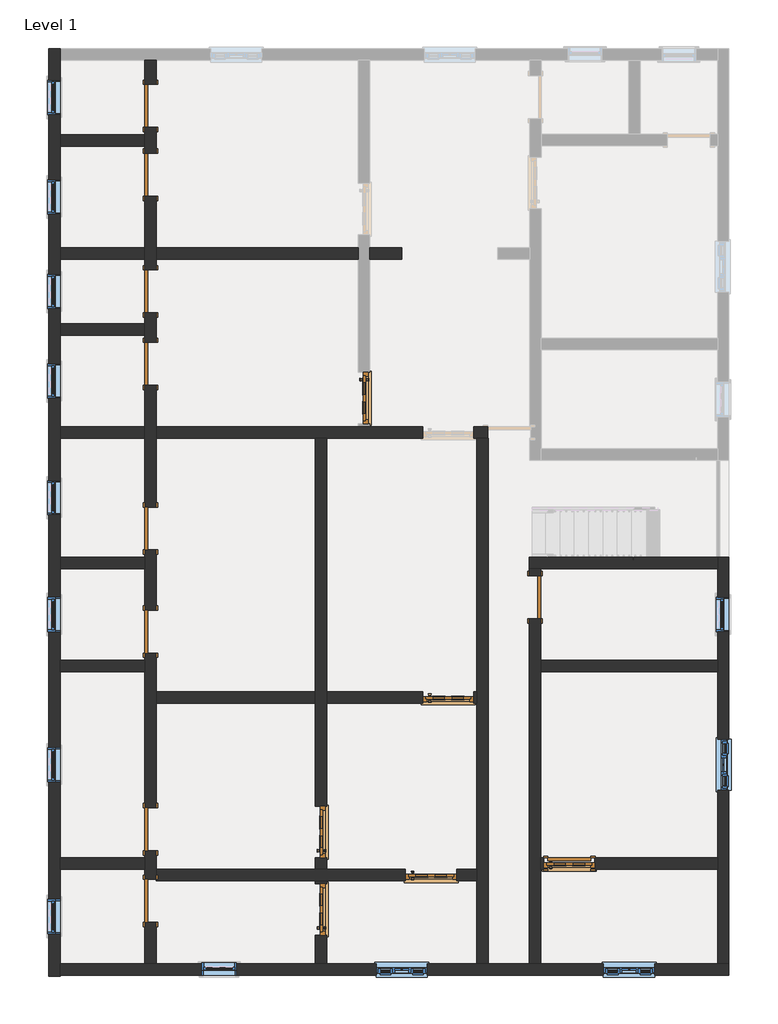
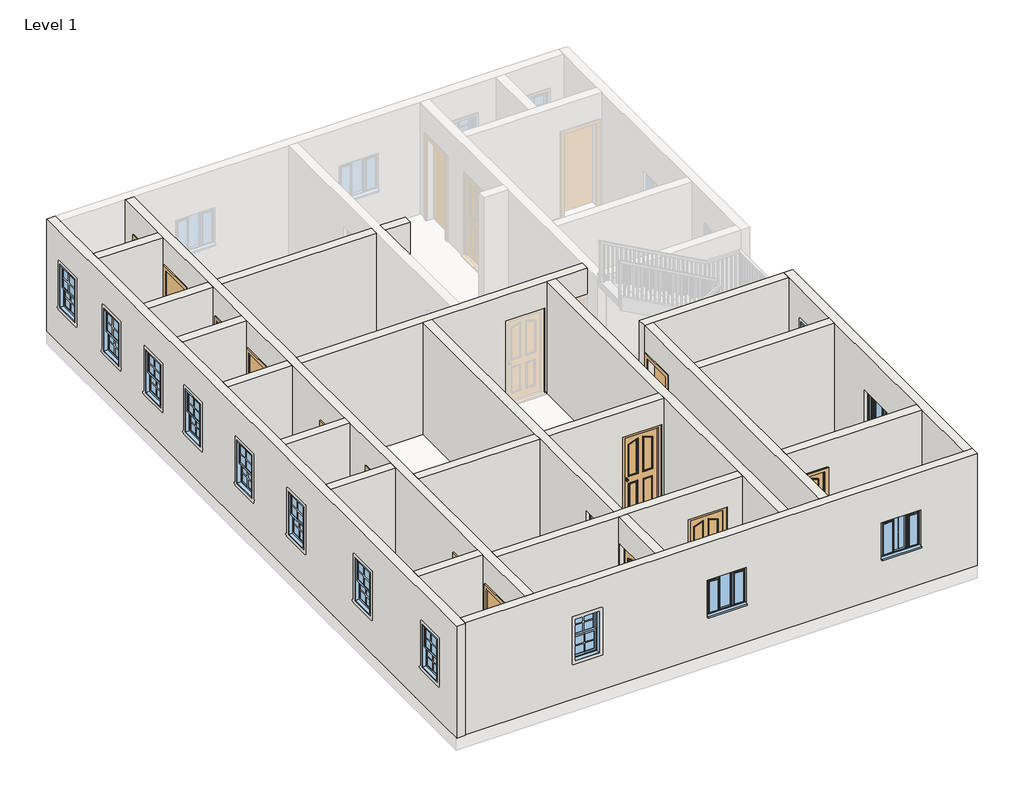
# One storey, part 1 of 3: 20 walls, 16 doors, 13 windows.
"""IFC4 building model written with IfcOpenShell, lengths in millimetres."""

from ifc_helpers import new_model, si_unit, frame, origin, origin_with_axes, place, context, project, spatial, polyline, outline, extrude, faceted_brep, transform, mapped, element, save
from components import doors_extsgl_12_910x2110mm_9a09825e, doors_extsgl_12_910x2110mm_ece77ece, door_fadea3f2, door_53b1b562, window_679d2811, windows_tpl_w_glazing_cross_bars_910x910mm_4aa0f884

model = new_model("IFC4")

# Units and contexts
model_context = context("Model", 3, world=origin())
ifc_project = project(units=[si_unit("LENGTHUNIT", "METRE", prefix="MILLI")], contexts=[model_context])

# Site, building, storey
site = spatial("IfcSite", under=ifc_project)
building = spatial("IfcBuilding", under=site)
storey = spatial("IfcBuildingStorey", under=building, Name="Level 1", Elevation=0.0)

# Doors
placement = place(None, origin())
doors_extsgl_12_910x2110mm_shape = doors_extsgl_12_910x2110mm_9a09825e(model_context)
element("IfcDoor", 1, ObjectType="Doors_ExtSgl_12 : 910x2110mm", at=placement, inside=storey, context=model_context, shape_type="MappedRepresentation", body=[
    mapped(doors_extsgl_12_910x2110mm_shape, transform((-4887.6876145, 1213.3404944, 0.0), x_axis=(0.0, -1.0, 0.0), y_axis=(1.0, 0.0, 0.0), z_axis=(0.0, 0.0, 1.0))),
])
doors_extsgl_12_910x2110mm_2_shape = doors_extsgl_12_910x2110mm_ece77ece(model_context)
element("IfcDoor", 2, ObjectType="Doors_ExtSgl_12 : 910x2110mm", at=placement, inside=storey, context=model_context, shape_type="MappedRepresentation", body=[
    mapped(doors_extsgl_12_910x2110mm_2_shape, transform((-5649.6876145, -6482.8595056, 0.0), x_axis=(0.0, 1.0, 0.0), y_axis=(-1.0, 0.0, 0.0), z_axis=(0.0, 0.0, 1.0))),
])
element("IfcDoor", 3, ObjectType="Doors_ExtSgl_12 : 910x2110mm", at=placement, inside=storey, context=model_context, shape_type="MappedRepresentation", body=[
    mapped(doors_extsgl_12_910x2110mm_2_shape, transform((-1242.7876145, -7041.6595056, 0.0), x_axis=(1.0, 0.0, 0.0), y_axis=(0.0, 1.0, 0.0), z_axis=(0.0, 0.0, 1.0))),
])
element("IfcDoor", 4, ObjectType="Doors_ExtSgl_12 : 910x2110mm", at=placement, inside=storey, context=model_context, shape_type="MappedRepresentation", body=[
    mapped(doors_extsgl_12_910x2110mm_2_shape, transform((-5649.6876145, -7854.4595056, 0.0), x_axis=(0.0, 1.0, 0.0), y_axis=(-1.0, 0.0, 0.0), z_axis=(0.0, 0.0, 1.0))),
])
element("IfcDoor", 5, ObjectType="Doors_ExtSgl_12 : 910x2110mm", at=placement, inside=storey, context=model_context, shape_type="MappedRepresentation", body=[
    mapped(doors_extsgl_12_910x2110mm_2_shape, transform((-3693.8876145, -7244.8595056, 0.0), x_axis=(1.0, 0.0, 0.0), y_axis=(0.0, 1.0, 0.0), z_axis=(0.0, 0.0, 1.0))),
])
element("IfcDoor", 6, ObjectType="Doors_ExtSgl_12 : 910x2110mm", at=placement, inside=storey, context=model_context, shape_type="MappedRepresentation", body=[
    mapped(doors_extsgl_12_910x2110mm_2_shape, transform((-3389.0876145, -4095.2595056, 0.0), x_axis=(1.0, 0.0, 0.0), y_axis=(0.0, 1.0, 0.0), z_axis=(0.0, 0.0, 1.0))),
])
door_shape = door_fadea3f2(model_context)
element("IfcDoor", 7, ObjectType="Single-Flush : 30\" x 80\"", at=placement, inside=storey, context=model_context, shape_type="MappedRepresentation", body=[
    mapped(door_shape, transform((-8672.2876145, 5175.7404944, 0.0), x_axis=(0.0, 1.0, 0.0), y_axis=(-1.0, 0.0, 0.0), z_axis=(0.0, 0.0, 1.0))),
])
element("IfcDoor", 8, ObjectType="Single-Flush : 30\" x 80\"", at=placement, inside=storey, context=model_context, shape_type="MappedRepresentation", body=[
    mapped(door_shape, transform((-8672.2876145, -7702.0595056, 0.0), x_axis=(0.0, 1.0, 0.0), y_axis=(-1.0, 0.0, 0.0), z_axis=(0.0, 0.0, 1.0))),
])
element("IfcDoor", 9, ObjectType="Single-Flush : 30\" x 80\"", at=placement, inside=storey, context=model_context, shape_type="MappedRepresentation", body=[
    mapped(door_shape, transform((-1852.3876145, -2317.2595056, 0.0), x_axis=(0.0, -1.0, 0.0), y_axis=(1.0, 0.0, 0.0), z_axis=(0.0, 0.0, 1.0))),
])
element("IfcDoor", 10, ObjectType="Single-Flush : 30\" x 80\"", at=placement, inside=storey, context=model_context, shape_type="MappedRepresentation", body=[
    mapped(door_shape, transform((-1242.7876145, -7041.6595056, 0.0), x_axis=(1.0, 0.0, 0.0), y_axis=(0.0, 1.0, 0.0), z_axis=(0.0, 0.0, 1.0))),
])
door_2_shape = door_53b1b562(model_context)
element("IfcDoor", 11, ObjectType="Single-Flush : 30\" x 80\"", at=placement, inside=storey, context=model_context, shape_type="MappedRepresentation", body=[
    mapped(door_2_shape, transform((-8672.2876145, 6394.9404944, 0.0), x_axis=(0.0, -1.0, 0.0), y_axis=(1.0, 0.0, 0.0), z_axis=(0.0, 0.0, 1.0))),
])
element("IfcDoor", 12, ObjectType="Single-Flush : 30\" x 80\"", at=placement, inside=storey, context=model_context, shape_type="MappedRepresentation", body=[
    mapped(door_2_shape, transform((-8672.2876145, 3105.6404944, 0.0), x_axis=(0.0, -1.0, 0.0), y_axis=(1.0, 0.0, 0.0), z_axis=(0.0, 0.0, 1.0))),
])
element("IfcDoor", 13, ObjectType="Single-Flush : 30\" x 80\"", at=placement, inside=storey, context=model_context, shape_type="MappedRepresentation", body=[
    mapped(door_2_shape, transform((-8672.2876145, 1822.9404944, 0.0), x_axis=(0.0, -1.0, 0.0), y_axis=(1.0, 0.0, 0.0), z_axis=(0.0, 0.0, 1.0))),
])
element("IfcDoor", 14, ObjectType="Single-Flush : 30\" x 80\"", at=placement, inside=storey, context=model_context, shape_type="MappedRepresentation", body=[
    mapped(door_2_shape, transform((-8672.2876145, -1098.0595056, 0.0), x_axis=(0.0, -1.0, 0.0), y_axis=(1.0, 0.0, 0.0), z_axis=(0.0, 0.0, 1.0))),
])
element("IfcDoor", 15, ObjectType="Single-Flush : 30\" x 80\"", at=placement, inside=storey, context=model_context, shape_type="MappedRepresentation", body=[
    mapped(door_2_shape, transform((-8672.2876145, -2926.8595056, 0.0), x_axis=(0.0, -1.0, 0.0), y_axis=(1.0, 0.0, 0.0), z_axis=(0.0, 0.0, 1.0))),
])
element("IfcDoor", 16, ObjectType="Single-Flush : 30\" x 80\"", at=placement, inside=storey, context=model_context, shape_type="MappedRepresentation", body=[
    mapped(door_2_shape, transform((-8672.2876145, -6432.0595056, 0.0), x_axis=(0.0, -1.0, 0.0), y_axis=(1.0, 0.0, 0.0), z_axis=(0.0, 0.0, 1.0))),
])

# Walls
element("IfcWall", 17, ObjectType="4.5\"", at=placement, inside=storey, context=model_context, shape_type="Brep", body=[
    faceted_brep([(-8773.8876145, -6813.0595056, 0.0), (-8773.8876145, -6940.0595056, 0.0), (-8773.8876145, -7143.2595056, 0.0), (-8773.8876145, -7321.0595056, 0.0), (-8773.8876145, -7321.0595056, 2032.0), (-8773.8876145, -8083.0595056, 2032.0), (-8773.8876145, -8083.0595056, 0.0), (-8773.8876145, -8819.6595056, 0.0), (-8773.8876145, -8819.6595056, 2743.2), (-8773.8876145, -7143.2595056, 2743.2), (-8773.8876145, -6940.0595056, 2743.2), (-8773.8876145, -3638.0595056, 2743.2), (-8773.8876145, -3434.8595056, 2743.2), (-8773.8876145, -1809.2595056, 2743.2), (-8773.8876145, -1606.0595056, 2743.2), (-8773.8876145, 502.1404944, 2743.2), (-8773.8876145, 705.3404944, 2743.2), (-8773.8876145, 2330.9404944, 2743.2), (-8773.8876145, 2534.1404944, 2743.2), (-8773.8876145, 3677.1404944, 2743.2), (-8773.8876145, 3880.3404944, 2743.2), (-8773.8876145, 5683.7404944, 2743.2), (-8773.8876145, 5886.9404944, 2743.2), (-8773.8876145, 7207.7404944, 2743.2), (-8773.8876145, 7207.7404944, 0.0), (-8773.8876145, 6775.9404944, 0.0), (-8773.8876145, 6775.9404944, 2032.0), (-8773.8876145, 6013.9404944, 2032.0), (-8773.8876145, 6013.9404944, 0.0), (-8773.8876145, 5886.9404944, 0.0), (-8773.8876145, 5683.7404944, 0.0), (-8773.8876145, 5556.7404944, 0.0), (-8773.8876145, 5556.7404944, 2032.0), (-8773.8876145, 4794.7404944, 2032.0), (-8773.8876145, 4794.7404944, 0.0), (-8773.8876145, 3880.3404944, 0.0), (-8773.8876145, 3677.1404944, 0.0), (-8773.8876145, 3486.6404944, 0.0), (-8773.8876145, 3486.6404944, 2032.0), (-8773.8876145, 2724.6404944, 2032.0), (-8773.8876145, 2724.6404944, 0.0), (-8773.8876145, 2534.1404944, 0.0), (-8773.8876145, 2330.9404944, 0.0), (-8773.8876145, 2203.9404944, 0.0), (-8773.8876145, 2203.9404944, 2032.0), (-8773.8876145, 1441.9404944, 2032.0), (-8773.8876145, 1441.9404944, 0.0), (-8773.8876145, 705.3404944, 0.0), (-8773.8876145, 502.1404944, 0.0), (-8773.8876145, -717.0595056, 0.0), (-8773.8876145, -717.0595056, 2032.0), (-8773.8876145, -1479.0595056, 2032.0), (-8773.8876145, -1479.0595056, 0.0), (-8773.8876145, -1606.0595056, 0.0), (-8773.8876145, -1809.2595056, 0.0), (-8773.8876145, -2545.8595056, 0.0), (-8773.8876145, -2545.8595056, 2032.0), (-8773.8876145, -3307.8595056, 2032.0), (-8773.8876145, -3307.8595056, 0.0), (-8773.8876145, -3434.8595056, 0.0), (-8773.8876145, -3638.0595056, 0.0), (-8773.8876145, -6051.0595056, 0.0), (-8773.8876145, -6051.0595056, 2032.0), (-8773.8876145, -6813.0595056, 2032.0), (-8570.6876145, -7321.0595056, 2032.0), (-8570.6876145, -7321.0595056, 0.0), (-8570.6876145, -7143.2595056, 0.0), (-8570.6876145, -6813.0595056, 0.0), (-8570.6876145, -6813.0595056, 2032.0), (-8570.6876145, -6051.0595056, 2032.0), (-8570.6876145, -6051.0595056, 0.0), (-8570.6876145, -4196.8595056, 0.0), (-8570.6876145, -3993.6595056, 0.0), (-8570.6876145, -3307.8595056, 0.0), (-8570.6876145, -3307.8595056, 2032.0), (-8570.6876145, -2545.8595056, 2032.0), (-8570.6876145, -2545.8595056, 0.0), (-8570.6876145, -1479.0595056, 0.0), (-8570.6876145, -1479.0595056, 2032.0), (-8570.6876145, -717.0595056, 2032.0), (-8570.6876145, -717.0595056, 0.0), (-8570.6876145, 502.1404944, 0.0), (-8570.6876145, 705.3404944, 0.0), (-8570.6876145, 1441.9404944, 0.0), (-8570.6876145, 1441.9404944, 2032.0), (-8570.6876145, 2203.9404944, 2032.0), (-8570.6876145, 2203.9404944, 0.0), (-8570.6876145, 2724.6404944, 0.0), (-8570.6876145, 2724.6404944, 2032.0), (-8570.6876145, 3486.6404944, 2032.0), (-8570.6876145, 3486.6404944, 0.0), (-8570.6876145, 3677.1404944, 0.0), (-8570.6876145, 3880.3404944, 0.0), (-8570.6876145, 4794.7404944, 0.0), (-8570.6876145, 4794.7404944, 2032.0), (-8570.6876145, 5556.7404944, 2032.0), (-8570.6876145, 5556.7404944, 0.0), (-8570.6876145, 6013.9404944, 0.0), (-8570.6876145, 6013.9404944, 2032.0), (-8570.6876145, 6775.9404944, 2032.0), (-8570.6876145, 6775.9404944, 0.0), (-8570.6876145, 7207.7404944, 0.0), (-8570.6876145, 7207.7404944, 2743.2), (-8570.6876145, 3880.3404944, 2743.2), (-8570.6876145, 3677.1404944, 2743.2), (-8570.6876145, 705.3404944, 2743.2), (-8570.6876145, 502.1404944, 2743.2), (-8570.6876145, -3993.6595056, 2743.2), (-8570.6876145, -4196.8595056, 2743.2), (-8570.6876145, -7143.2595056, 2743.2), (-8570.6876145, -7346.4595056, 2743.2), (-8570.6876145, -8819.6595056, 2743.2), (-8570.6876145, -8819.6595056, 0.0), (-8570.6876145, -8083.0595056, 0.0), (-8570.6876145, -8083.0595056, 2032.0)], [[[0, 1, 2, 3, 4, 5, 6, 7, 8, 9, 10, 11, 12, 13, 14, 15, 16, 17, 18, 19, 20, 21, 22, 23, 24, 25, 26, 27, 28, 29, 30, 31, 32, 33, 34, 35, 36, 37, 38, 39, 40, 41, 42, 43, 44, 45, 46, 47, 48, 49, 50, 51, 52, 53, 54, 55, 56, 57, 58, 59, 60, 61, 62, 63]], [[64, 65, 66, 67, 68, 69, 70, 71, 72, 73, 74, 75, 76, 77, 78, 79, 80, 81, 82, 83, 84, 85, 86, 87, 88, 89, 90, 91, 92, 93, 94, 95, 96, 97, 98, 99, 100, 101, 102, 103, 104, 105, 106, 107, 108, 109, 110, 111, 112, 113, 114]], [[25, 24, 101, 100]], [[97, 96, 31, 30, 29, 28]], [[37, 36, 35, 34, 93, 92, 91, 90]], [[43, 42, 41, 40, 87, 86]], [[49, 48, 47, 46, 83, 82, 81, 80]], [[55, 54, 53, 52, 77, 76]], [[61, 60, 59, 58, 73, 72, 71, 70]], [[113, 112, 7, 6]], [[67, 66, 65, 3, 2, 1, 0]], [[8, 7, 112, 111]], [[24, 23, 102, 101]], [[98, 97, 28, 27]], [[99, 98, 27, 26]], [[100, 99, 26, 25]], [[32, 31, 96, 95]], [[33, 32, 95, 94]], [[34, 33, 94, 93]], [[88, 87, 40, 39]], [[89, 88, 39, 38]], [[90, 89, 38, 37]], [[84, 83, 46, 45]], [[85, 84, 45, 44]], [[86, 85, 44, 43]], [[78, 77, 52, 51]], [[79, 78, 51, 50]], [[80, 79, 50, 49]], [[74, 73, 58, 57]], [[75, 74, 57, 56]], [[76, 75, 56, 55]], [[68, 67, 0, 63]], [[69, 68, 63, 62]], [[70, 69, 62, 61]], [[4, 3, 65, 64]], [[5, 4, 64, 114]], [[6, 5, 114, 113]], [[23, 22, 21, 20, 19, 18, 17, 16, 15, 14, 13, 12, 11, 10, 9, 8, 111, 110, 109, 108, 107, 106, 105, 104, 103, 102]]]),
])
element("IfcWall", 18, ObjectType="4.5\"", at=placement, inside=storey, context=model_context, shape_type="SweptSolid", body=[
    extrude(outline(polyline([(-8773.8876145, 5683.7404944), (-10272.4876145, 5683.7404944), (-10272.4876145, 5886.9404944), (-8773.8876145, 5886.9404944), (-8773.8876145, 5683.7404944)])), origin_with_axes(), (0.0, 0.0, 1.0), 2743.2),
])
element("IfcWall", 19, ObjectType="4.5\"", at=placement, inside=storey, context=model_context, shape_type="SweptSolid", body=[
    extrude(outline(polyline([(-8773.8876145, 3677.1404944), (-10272.4876145, 3677.1404944), (-10272.4876145, 3880.3404944), (-8773.8876145, 3880.3404944), (-8773.8876145, 3677.1404944)])), origin_with_axes(), (0.0, 0.0, 1.0), 2743.2),
])
element("IfcWall", 20, ObjectType="4.5\"", at=placement, inside=storey, context=model_context, shape_type="SweptSolid", body=[
    extrude(outline(polyline([(-8773.8876145, 2330.9404944), (-10272.4876145, 2330.9404944), (-10272.4876145, 2534.1404944), (-8773.8876145, 2534.1404944), (-8773.8876145, 2330.9404944)])), origin_with_axes(), (0.0, 0.0, 1.0), 2743.2),
])
element("IfcWall", 21, ObjectType="4.5\"", at=placement, inside=storey, context=model_context, shape_type="Brep", body=[
    faceted_brep([(-10272.4876145, 502.1404944, 2743.2), (-10272.4876145, 502.1404944, 0.0), (-8773.8876145, 502.1404944, 0.0), (-8773.8876145, 502.1404944, 2743.2), (-10272.4876145, 705.3404944, 0.0), (-10272.4876145, 705.3404944, 2743.2), (-8773.8876145, 705.3404944, 2743.2), (-8773.8876145, 705.3404944, 0.0)], [[[0, 1, 2, 3]], [[4, 5, 6, 7]], [[1, 4, 7, 2]], [[1, 0, 5, 4]], [[3, 2, 7, 6]], [[5, 0, 3, 6]]]),
    faceted_brep([(-1941.2876145, 502.1404944, 2032.0), (-1941.2876145, 502.1404944, 2743.2), (-2677.8876145, 502.1404944, 2743.2), (-2881.0876145, 502.1404944, 2743.2), (-5548.0876145, 502.1404944, 2743.2), (-5751.2876145, 502.1404944, 2743.2), (-8570.6876145, 502.1404944, 2743.2), (-8570.6876145, 502.1404944, 0.0), (-5751.2876145, 502.1404944, 0.0), (-5548.0876145, 502.1404944, 0.0), (-3844.0876145, 502.1404944, 0.0), (-3844.0876145, 502.1404944, 2110.0), (-2934.0876145, 502.1404944, 2110.0), (-2934.0876145, 502.1404944, 0.0), (-2881.0876145, 502.1404944, 0.0), (-2690.5876145, 502.1404944, 0.0), (-2690.5876145, 502.1404944, 2032.0), (-1941.2876145, 705.3404944, 2743.2), (-1941.2876145, 705.3404944, 2032.0), (-2690.5876145, 705.3404944, 2032.0), (-2690.5876145, 705.3404944, 0.0), (-2934.0876145, 705.3404944, 0.0), (-2934.0876145, 705.3404944, 2110.0), (-3844.0876145, 705.3404944, 2110.0), (-3844.0876145, 705.3404944, 0.0), (-4786.0876145, 705.3404944, 0.0), (-4989.2876145, 705.3404944, 0.0), (-8570.6876145, 705.3404944, 0.0), (-8570.6876145, 705.3404944, 2743.2), (-4989.2876145, 705.3404944, 2743.2), (-4786.0876145, 705.3404944, 2743.2)], [[[0, 1, 2, 3, 4, 5, 6, 7, 8, 9, 10, 11, 12, 13, 14, 15, 16]], [[17, 18, 19, 20, 21, 22, 23, 24, 25, 26, 27, 28, 29, 30]], [[20, 15, 14, 13, 21]], [[24, 10, 9, 8, 7, 27, 26, 25]], [[7, 6, 28, 27]], [[1, 0, 18, 17]], [[16, 19, 18, 0]], [[19, 16, 15, 20]], [[24, 23, 11, 10]], [[22, 21, 13, 12]], [[23, 22, 12, 11]], [[1, 17, 30, 29, 28, 6, 5, 4, 3, 2]]]),
])
element("IfcWall", 22, ObjectType="4.5\"", at=placement, inside=storey, context=model_context, shape_type="SweptSolid", body=[
    extrude(outline(polyline([(-8773.8876145, -1809.2595056), (-10272.4876145, -1809.2595056), (-10272.4876145, -1606.0595056), (-8773.8876145, -1606.0595056), (-8773.8876145, -1809.2595056)])), origin_with_axes(), (0.0, 0.0, 1.0), 2743.2),
])
element("IfcWall", 23, ObjectType="4.5\"", at=placement, inside=storey, context=model_context, shape_type="SweptSolid", body=[
    extrude(outline(polyline([(-8773.8876145, -3638.0595056), (-10272.4876145, -3638.0595056), (-10272.4876145, -3434.8595056), (-8773.8876145, -3434.8595056), (-8773.8876145, -3638.0595056)])), origin_with_axes(), (0.0, 0.0, 1.0), 2743.2),
])
element("IfcWall", 24, ObjectType="4.5\"", at=placement, inside=storey, context=model_context, shape_type="SweptSolid", body=[
    extrude(outline(polyline([(-8773.8876145, -7143.2595056), (-10272.4876145, -7143.2595056), (-10272.4876145, -6940.0595056), (-8773.8876145, -6940.0595056), (-8773.8876145, -7143.2595056)])), origin_with_axes(), (0.0, 0.0, 1.0), 2743.2),
])
element("IfcWall", 25, ObjectType="4.5\"", at=placement, inside=storey, context=model_context, shape_type="Brep", body=[
    faceted_brep([(-3238.8876145, -7346.4595056, 2110.0), (-3238.8876145, -7346.4595056, 0.0), (-2881.0876145, -7346.4595056, 0.0), (-2881.0876145, -7346.4595056, 2743.2), (-5548.0876145, -7346.4595056, 2743.2), (-5751.2876145, -7346.4595056, 2743.2), (-8570.6876145, -7346.4595056, 2743.2), (-8570.6876145, -7346.4595056, 0.0), (-5751.2876145, -7346.4595056, 0.0), (-5548.0876145, -7346.4595056, 0.0), (-4148.8876145, -7346.4595056, 0.0), (-4148.8876145, -7346.4595056, 2110.0), (-2881.0876145, -7143.2595056, 0.0), (-3238.8876145, -7143.2595056, 0.0), (-3238.8876145, -7143.2595056, 2110.0), (-4148.8876145, -7143.2595056, 2110.0), (-4148.8876145, -7143.2595056, 0.0), (-5548.0876145, -7143.2595056, 0.0), (-5751.2876145, -7143.2595056, 0.0), (-8570.6876145, -7143.2595056, 0.0), (-8570.6876145, -7143.2595056, 2743.2), (-5751.2876145, -7143.2595056, 2743.2), (-5548.0876145, -7143.2595056, 2743.2), (-2881.0876145, -7143.2595056, 2743.2), (-8570.6876145, -7321.0595056, 0.0)], [[[0, 1, 2, 3, 4, 5, 6, 7, 8, 9, 10, 11]], [[12, 13, 14, 15, 16, 17, 18, 19, 20, 21, 22, 23]], [[2, 1, 13, 12]], [[10, 9, 8, 7, 24, 19, 18, 17, 16]], [[7, 6, 20, 19, 24]], [[3, 2, 12, 23]], [[16, 15, 11, 10]], [[14, 13, 1, 0]], [[15, 14, 0, 11]], [[6, 5, 4, 3, 23, 22, 21, 20]]]),
])
element("IfcWall", 26, ObjectType="4.5\"", at=placement, inside=storey, context=model_context, shape_type="Brep", body=[
    faceted_brep([(-5751.2876145, -8819.6595056, 0.0), (-5751.2876145, -8819.6595056, 2743.2), (-5751.2876145, -7346.4595056, 2743.2), (-5751.2876145, -7346.4595056, 0.0), (-5751.2876145, -7399.4595056, 0.0), (-5751.2876145, -7399.4595056, 2110.0), (-5751.2876145, -8309.4595056, 2110.0), (-5751.2876145, -8309.4595056, 0.0), (-5548.0876145, -8819.6595056, 2743.2), (-5548.0876145, -8819.6595056, 0.0), (-5548.0876145, -8309.4595056, 0.0), (-5548.0876145, -8309.4595056, 2110.0), (-5548.0876145, -7399.4595056, 2110.0), (-5548.0876145, -7399.4595056, 0.0), (-5548.0876145, -7346.4595056, 0.0), (-5548.0876145, -7346.4595056, 2743.2)], [[[0, 1, 2, 3, 4, 5, 6, 7]], [[8, 9, 10, 11, 12, 13, 14, 15]], [[9, 0, 7, 10]], [[13, 4, 3, 14]], [[1, 0, 9, 8]], [[3, 2, 15, 14]], [[7, 6, 11, 10]], [[5, 4, 13, 12]], [[6, 5, 12, 11]], [[1, 8, 15, 2]]]),
    faceted_brep([(-5751.2876145, 502.1404944, 2743.2), (-5751.2876145, 502.1404944, 0.0), (-5751.2876145, -3993.6595056, 0.0), (-5751.2876145, -4196.8595056, 0.0), (-5751.2876145, -6027.8595056, 0.0), (-5751.2876145, -6027.8595056, 2110.0), (-5751.2876145, -6937.8595056, 2110.0), (-5751.2876145, -6937.8595056, 0.0), (-5751.2876145, -7143.2595056, 0.0), (-5751.2876145, -7143.2595056, 2743.2), (-5751.2876145, -4196.8595056, 2743.2), (-5751.2876145, -3993.6595056, 2743.2), (-5548.0876145, 502.1404944, 0.0), (-5548.0876145, 502.1404944, 2743.2), (-5548.0876145, -3993.6595056, 2743.2), (-5548.0876145, -4196.8595056, 2743.2), (-5548.0876145, -7143.2595056, 2743.2), (-5548.0876145, -7143.2595056, 0.0), (-5548.0876145, -6937.8595056, 0.0), (-5548.0876145, -6937.8595056, 2110.0), (-5548.0876145, -6027.8595056, 2110.0), (-5548.0876145, -6027.8595056, 0.0), (-5548.0876145, -4196.8595056, 0.0), (-5548.0876145, -3993.6595056, 0.0)], [[[0, 1, 2, 3, 4, 5, 6, 7, 8, 9, 10, 11]], [[12, 13, 14, 15, 16, 17, 18, 19, 20, 21, 22, 23]], [[1, 12, 23, 22, 21, 4, 3, 2]], [[7, 18, 17, 8]], [[1, 0, 13, 12]], [[9, 8, 17, 16]], [[7, 6, 19, 18]], [[5, 4, 21, 20]], [[6, 5, 20, 19]], [[13, 0, 11, 10, 9, 16, 15, 14]]]),
])
element("IfcWall", 27, ObjectType="4.5\"", at=placement, inside=storey, context=model_context, shape_type="SweptSolid", body=[
    extrude(outline(polyline([(-8570.6876145, -4196.8595056), (-8570.6876145, -3993.6595056), (-5751.2876145, -3993.6595056), (-5751.2876145, -4196.8595056), (-8570.6876145, -4196.8595056)])), origin_with_axes(), (0.0, 0.0, 1.0), 2743.2),
    extrude(outline(polyline([(0.0, -2881.0876145), (2743.2, -2881.0876145), (2743.2, -5548.0876145), (0.0, -5548.0876145), (0.0, -3844.0876145), (2110.0, -3844.0876145), (2110.0, -2934.0876145), (0.0, -2934.0876145), (0.0, -2881.0876145)])), frame((0.0, -4196.8595056, 0.0), z_axis=(0.0, 1.0, 0.0), x_axis=(0.0, 0.0, 1.0)), (0.0, 0.0, 1.0), 203.2),
])
element("IfcWall", 28, ObjectType="4.5\"", at=placement, inside=storey, context=model_context, shape_type="Brep", body=[
    faceted_brep([(-2881.0876145, 502.1404944, 0.0), (-2881.0876145, -3993.6595056, 0.0), (-2881.0876145, -4196.8595056, 0.0), (-2881.0876145, -7143.2595056, 0.0), (-2881.0876145, -7346.4595056, 0.0), (-2881.0876145, -8819.6595056, 0.0), (-2881.0876145, -8819.6595056, 2743.2), (-2881.0876145, -7346.4595056, 2743.2), (-2881.0876145, -7143.2595056, 2743.2), (-2881.0876145, -4196.8595056, 2743.2), (-2881.0876145, -3993.6595056, 2743.2), (-2881.0876145, 502.1404944, 2743.2), (-2677.8876145, 502.1404944, 0.0), (-2677.8876145, 502.1404944, 2743.2), (-2677.8876145, -8819.6595056, 2743.2), (-2677.8876145, -8819.6595056, 0.0), (-2690.5876145, 502.1404944, 0.0)], [[[0, 1, 2, 3, 4, 5, 6, 7, 8, 9, 10, 11]], [[12, 13, 14, 15]], [[5, 4, 3, 2, 1, 0, 16, 12, 15]], [[6, 5, 15, 14]], [[0, 11, 13, 12, 16]], [[11, 10, 9, 8, 7, 6, 14, 13]]]),
])
element("IfcWall", 29, ObjectType="4.5\"", at=placement, inside=storey, context=model_context, shape_type="SweptSolid", body=[
    extrude(outline(polyline([(-4214.5876145, 3880.3404944), (-4214.5876145, 3677.1404944), (-4786.0876145, 3677.1404944), (-4786.0876145, 3880.3404944), (-4214.5876145, 3880.3404944)])), origin_with_axes(), (0.0, 0.0, 1.0), 2743.2),
    extrude(outline(polyline([(-8570.6876145, 3677.1404944), (-8570.6876145, 3880.3404944), (-4989.2876145, 3880.3404944), (-4989.2876145, 3677.1404944), (-8570.6876145, 3677.1404944)])), origin_with_axes(), (0.0, 0.0, 1.0), 2743.2),
])
element("IfcWall", 30, ObjectType="4.5\"", at=placement, inside=storey, context=model_context, shape_type="Brep", body=[
    faceted_brep([(1386.1123855, -1606.0595056, 0.0), (-1953.9876145, -1606.0595056, 0.0), (-1953.9876145, -1606.0595056, 2743.2), (1386.1123855, -1606.0595056, 2743.2), (1386.1123855, -1809.2595056, 0.0), (1386.1123855, -1809.2595056, 2743.2), (-1750.7876145, -1809.2595056, 2743.2), (-1953.9876145, -1809.2595056, 2743.2), (-1953.9876145, -1809.2595056, 0.0), (-1750.7876145, -1809.2595056, 0.0)], [[[0, 1, 2, 3]], [[4, 5, 6, 7, 8, 9]], [[1, 0, 4, 9, 8]], [[0, 3, 5, 4]], [[2, 1, 8, 7]], [[3, 2, 7, 6, 5]]]),
])
element("IfcWall", 31, ObjectType="4.5\"", at=placement, inside=storey, context=model_context, shape_type="Brep", body=[
    faceted_brep([(-1953.9876145, -2698.2595056, 2032.0), (-1953.9876145, -2698.2595056, 0.0), (-1953.9876145, -8819.6595056, 0.0), (-1953.9876145, -8819.6595056, 2743.2), (-1953.9876145, -1809.2595056, 2743.2), (-1953.9876145, -1809.2595056, 0.0), (-1953.9876145, -1936.2595056, 0.0), (-1953.9876145, -1936.2595056, 2032.0), (-1750.7876145, -8819.6595056, 0.0), (-1750.7876145, -7143.2595056, 0.0), (-1750.7876145, -6940.0595056, 0.0), (-1750.7876145, -3638.0595056, 0.0), (-1750.7876145, -3434.8595056, 0.0), (-1750.7876145, -2698.2595056, 0.0), (-1750.7876145, -2698.2595056, 2032.0), (-1750.7876145, -1936.2595056, 2032.0), (-1750.7876145, -1936.2595056, 0.0), (-1750.7876145, -1809.2595056, 0.0), (-1750.7876145, -1809.2595056, 2743.2), (-1750.7876145, -3434.8595056, 2743.2), (-1750.7876145, -3638.0595056, 2743.2), (-1750.7876145, -6940.0595056, 2743.2), (-1750.7876145, -7143.2595056, 2743.2), (-1750.7876145, -8819.6595056, 2743.2)], [[[0, 1, 2, 3, 4, 5, 6, 7]], [[8, 9, 10, 11, 12, 13, 14, 15, 16, 17, 18, 19, 20, 21, 22, 23]], [[6, 5, 17, 16]], [[2, 1, 13, 12, 11, 10, 9, 8]], [[5, 4, 18, 17]], [[3, 2, 8, 23]], [[14, 13, 1, 0]], [[15, 14, 0, 7]], [[16, 15, 7, 6]], [[4, 3, 23, 22, 21, 20, 19, 18]]]),
])
element("IfcWall", 32, ObjectType="4.5\"", at=placement, inside=storey, context=model_context, shape_type="SweptSolid", body=[
    extrude(outline(polyline([(0.0, 1386.1123855), (2743.2, 1386.1123855), (2743.2, -1750.7876145), (0.0, -1750.7876145), (0.0, -1697.7876145), (2110.0, -1697.7876145), (2110.0, -787.7876145), (0.0, -787.7876145), (0.0, 1386.1123855)])), frame((0.0, -7143.2595056, 0.0), z_axis=(0.0, 1.0, 0.0), x_axis=(0.0, 0.0, 1.0)), (0.0, 0.0, 1.0), 203.2),
])
element("IfcWall", 33, ObjectType="4.5\"", at=placement, inside=storey, context=model_context, shape_type="SweptSolid", body=[
    extrude(outline(polyline([(1386.1123855, -3638.0595056), (-1750.7876145, -3638.0595056), (-1750.7876145, -3434.8595056), (1386.1123855, -3434.8595056), (1386.1123855, -3638.0595056)])), origin_with_axes(), (0.0, 0.0, 1.0), 2743.2),
])
element("IfcWall", 34, ObjectType="Generic - 9\"", at=placement, inside=storey, context=model_context, shape_type="Brep", body=[
    faceted_brep([(-10475.6876145, 7410.9404944, 0.0), (-10475.6876145, -9035.5595056, 0.0), (-10475.6876145, -9035.5595056, 2743.2), (-10475.6876145, 7410.9404944, 2743.2), (-10475.6876145, 6242.5404944, 1981.2), (-10475.6876145, 6242.5404944, 914.4), (-10475.6876145, 6852.1404944, 914.4), (-10475.6876145, 6852.1404944, 1981.2), (-10475.6876145, 4477.2404944, 1981.2), (-10475.6876145, 4477.2404944, 914.4), (-10475.6876145, 5086.8404944, 914.4), (-10475.6876145, 5086.8404944, 1981.2), (-10475.6876145, 2800.8404944, 1981.2), (-10475.6876145, 2800.8404944, 914.4), (-10475.6876145, 3410.4404944, 914.4), (-10475.6876145, 3410.4404944, 1981.2), (-10475.6876145, 1213.3404944, 1981.2), (-10475.6876145, 1213.3404944, 914.4), (-10475.6876145, 1822.9404944, 914.4), (-10475.6876145, 1822.9404944, 1981.2), (-10475.6876145, -856.7595056, 1981.2), (-10475.6876145, -856.7595056, 914.4), (-10475.6876145, -247.1595056, 914.4), (-10475.6876145, -247.1595056, 1981.2), (-10475.6876145, -2926.8595056, 1981.2), (-10475.6876145, -2926.8595056, 914.4), (-10475.6876145, -2317.2595056, 914.4), (-10475.6876145, -2317.2595056, 1981.2), (-10475.6876145, -5593.8595056, 1981.2), (-10475.6876145, -5593.8595056, 914.4), (-10475.6876145, -4984.2595056, 914.4), (-10475.6876145, -4984.2595056, 1981.2), (-10475.6876145, -8286.2595056, 1981.2), (-10475.6876145, -8286.2595056, 914.4), (-10475.6876145, -7676.6595056, 914.4), (-10475.6876145, -7676.6595056, 1981.2), (-10272.4876145, 7410.9404944, 0.0), (-10272.4876145, 7410.9404944, 2743.2), (-10272.4876145, 7207.7404944, 2743.2), (-10272.4876145, 5886.9404944, 2743.2), (-10272.4876145, 5683.7404944, 2743.2), (-10272.4876145, 3880.3404944, 2743.2), (-10272.4876145, 3677.1404944, 2743.2), (-10272.4876145, 2534.1404944, 2743.2), (-10272.4876145, 2330.9404944, 2743.2), (-10272.4876145, 705.3404944, 2743.2), (-10272.4876145, 502.1404944, 2743.2), (-10272.4876145, -1606.0595056, 2743.2), (-10272.4876145, -1809.2595056, 2743.2), (-10272.4876145, -3434.8595056, 2743.2), (-10272.4876145, -3638.0595056, 2743.2), (-10272.4876145, -6940.0595056, 2743.2), (-10272.4876145, -7143.2595056, 2743.2), (-10272.4876145, -8819.6595056, 2743.2), (-10272.4876145, -9022.8595056, 2743.2), (-10272.4876145, -9035.5595056, 2743.2), (-10272.4876145, -9035.5595056, 0.0), (-10272.4876145, -9022.8595056, 0.0), (-10272.4876145, -8819.6595056, 0.0), (-10272.4876145, -7143.2595056, 0.0), (-10272.4876145, -6940.0595056, 0.0), (-10272.4876145, -3638.0595056, 0.0), (-10272.4876145, -3434.8595056, 0.0), (-10272.4876145, -1809.2595056, 0.0), (-10272.4876145, -1606.0595056, 0.0), (-10272.4876145, 502.1404944, 0.0), (-10272.4876145, 705.3404944, 0.0), (-10272.4876145, 2330.9404944, 0.0), (-10272.4876145, 2534.1404944, 0.0), (-10272.4876145, 3677.1404944, 0.0), (-10272.4876145, 3880.3404944, 0.0), (-10272.4876145, 5683.7404944, 0.0), (-10272.4876145, 5886.9404944, 0.0), (-10272.4876145, 7207.7404944, 0.0), (-10272.4876145, 6242.5404944, 1981.2), (-10272.4876145, 6852.1404944, 1981.2), (-10272.4876145, 6852.1404944, 914.4), (-10272.4876145, 6242.5404944, 914.4), (-10272.4876145, 4477.2404944, 1981.2), (-10272.4876145, 5086.8404944, 1981.2), (-10272.4876145, 5086.8404944, 914.4), (-10272.4876145, 4477.2404944, 914.4), (-10272.4876145, 2800.8404944, 1981.2), (-10272.4876145, 3410.4404944, 1981.2), (-10272.4876145, 3410.4404944, 914.4), (-10272.4876145, 2800.8404944, 914.4), (-10272.4876145, 1213.3404944, 1981.2), (-10272.4876145, 1822.9404944, 1981.2), (-10272.4876145, 1822.9404944, 914.4), (-10272.4876145, 1213.3404944, 914.4), (-10272.4876145, -856.7595056, 1981.2), (-10272.4876145, -247.1595056, 1981.2), (-10272.4876145, -247.1595056, 914.4), (-10272.4876145, -856.7595056, 914.4), (-10272.4876145, -2926.8595056, 1981.2), (-10272.4876145, -2317.2595056, 1981.2), (-10272.4876145, -2317.2595056, 914.4), (-10272.4876145, -2926.8595056, 914.4), (-10272.4876145, -5593.8595056, 1981.2), (-10272.4876145, -4984.2595056, 1981.2), (-10272.4876145, -4984.2595056, 914.4), (-10272.4876145, -5593.8595056, 914.4), (-10272.4876145, -8286.2595056, 1981.2), (-10272.4876145, -7676.6595056, 1981.2), (-10272.4876145, -7676.6595056, 914.4), (-10272.4876145, -8286.2595056, 914.4)], [[[0, 1, 2, 3], [4, 5, 6, 7], [8, 9, 10, 11], [12, 13, 14, 15], [16, 17, 18, 19], [20, 21, 22, 23], [24, 25, 26, 27], [28, 29, 30, 31], [32, 33, 34, 35]], [[36, 37, 38, 39, 40, 41, 42, 43, 44, 45, 46, 47, 48, 49, 50, 51, 52, 53, 54, 55, 56, 57, 58, 59, 60, 61, 62, 63, 64, 65, 66, 67, 68, 69, 70, 71, 72, 73], [74, 75, 76, 77], [78, 79, 80, 81], [82, 83, 84, 85], [86, 87, 88, 89], [90, 91, 92, 93], [94, 95, 96, 97], [98, 99, 100, 101], [102, 103, 104, 105]], [[1, 0, 36, 73, 72, 71, 70, 69, 68, 67, 66, 65, 64, 63, 62, 61, 60, 59, 58, 57, 56]], [[2, 1, 56, 55]], [[0, 3, 37, 36]], [[5, 4, 74, 77]], [[6, 5, 77, 76]], [[7, 6, 76, 75]], [[4, 7, 75, 74]], [[9, 8, 78, 81]], [[10, 9, 81, 80]], [[11, 10, 80, 79]], [[8, 11, 79, 78]], [[13, 12, 82, 85]], [[14, 13, 85, 84]], [[15, 14, 84, 83]], [[12, 15, 83, 82]], [[17, 16, 86, 89]], [[18, 17, 89, 88]], [[19, 18, 88, 87]], [[16, 19, 87, 86]], [[21, 20, 90, 93]], [[22, 21, 93, 92]], [[23, 22, 92, 91]], [[20, 23, 91, 90]], [[25, 24, 94, 97]], [[26, 25, 97, 96]], [[27, 26, 96, 95]], [[24, 27, 95, 94]], [[29, 28, 98, 101]], [[30, 29, 101, 100]], [[31, 30, 100, 99]], [[28, 31, 99, 98]], [[33, 32, 102, 105]], [[34, 33, 105, 104]], [[35, 34, 104, 103]], [[32, 35, 103, 102]], [[3, 2, 55, 54, 53, 52, 51, 50, 49, 48, 47, 46, 45, 44, 43, 42, 41, 40, 39, 38, 37]]]),
])
element("IfcWall", 35, ObjectType="Generic - 9\"", at=placement, inside=storey, context=model_context, shape_type="Brep", body=[
    faceted_brep([(-10272.4876145, -9022.8595056, 0.0), (1589.3123855, -9022.8595056, 0.0), (1589.3123855, -9022.8595056, 2743.2), (-10272.4876145, -9022.8595056, 2743.2), (-7757.8876145, -9022.8595056, 1981.2), (-7148.2876145, -9022.8595056, 1981.2), (-7148.2876145, -9022.8595056, 914.4), (-7757.8876145, -9022.8595056, 914.4), (272.6623855, -9022.8595056, 1824.4), (272.6623855, -9022.8595056, 914.4), (-637.3376145, -9022.8595056, 914.4), (-637.3376145, -9022.8595056, 1824.4), (-3759.5876145, -9022.8595056, 1824.4), (-3759.5876145, -9022.8595056, 914.4), (-4669.5876145, -9022.8595056, 914.4), (-4669.5876145, -9022.8595056, 1824.4), (-10272.4876145, -8819.6595056, 0.0), (-10272.4876145, -8819.6595056, 2743.2), (-8773.8876145, -8819.6595056, 2743.2), (-8570.6876145, -8819.6595056, 2743.2), (-5751.2876145, -8819.6595056, 2743.2), (-5548.0876145, -8819.6595056, 2743.2), (-2881.0876145, -8819.6595056, 2743.2), (-2677.8876145, -8819.6595056, 2743.2), (-1953.9876145, -8819.6595056, 2743.2), (-1750.7876145, -8819.6595056, 2743.2), (1386.1123855, -8819.6595056, 2743.2), (1589.3123855, -8819.6595056, 2743.2), (1589.3123855, -8819.6595056, 0.0), (1386.1123855, -8819.6595056, 0.0), (-1750.7876145, -8819.6595056, 0.0), (-1953.9876145, -8819.6595056, 0.0), (-2677.8876145, -8819.6595056, 0.0), (-2881.0876145, -8819.6595056, 0.0), (-5548.0876145, -8819.6595056, 0.0), (-5751.2876145, -8819.6595056, 0.0), (-8570.6876145, -8819.6595056, 0.0), (-8773.8876145, -8819.6595056, 0.0), (-7757.8876145, -8819.6595056, 1981.2), (-7757.8876145, -8819.6595056, 914.4), (-7148.2876145, -8819.6595056, 914.4), (-7148.2876145, -8819.6595056, 1981.2), (272.6623855, -8819.6595056, 1824.4), (-637.3376145, -8819.6595056, 1824.4), (-637.3376145, -8819.6595056, 914.4), (272.6623855, -8819.6595056, 914.4), (-3759.5876145, -8819.6595056, 1824.4), (-4669.5876145, -8819.6595056, 1824.4), (-4669.5876145, -8819.6595056, 914.4), (-3759.5876145, -8819.6595056, 914.4)], [[[0, 1, 2, 3], [4, 5, 6, 7], [8, 9, 10, 11], [12, 13, 14, 15]], [[16, 17, 18, 19, 20, 21, 22, 23, 24, 25, 26, 27, 28, 29, 30, 31, 32, 33, 34, 35, 36, 37], [38, 39, 40, 41], [42, 43, 44, 45], [46, 47, 48, 49]], [[1, 0, 16, 37, 36, 35, 34, 33, 32, 31, 30, 29, 28]], [[0, 3, 17, 16]], [[2, 1, 28, 27]], [[39, 38, 4, 7]], [[40, 39, 7, 6]], [[41, 40, 6, 5]], [[38, 41, 5, 4]], [[9, 8, 42, 45]], [[10, 9, 45, 44]], [[11, 10, 44, 43]], [[8, 11, 43, 42]], [[13, 12, 46, 49]], [[14, 13, 49, 48]], [[15, 14, 48, 47]], [[12, 15, 47, 46]], [[3, 2, 27, 26, 25, 24, 23, 22, 21, 20, 19, 18, 17]]]),
])
element("IfcWall", 36, ObjectType="Generic - 9\"", at=placement, inside=storey, context=model_context, shape_type="Brep", body=[
    faceted_brep([(1589.3123855, -8819.6595056, 0.0), (1589.3123855, -1606.0595056, 0.0), (1589.3123855, -1606.0595056, 2743.2), (1589.3123855, -8819.6595056, 2743.2), (1589.3123855, -4834.0595056, 1824.4), (1589.3123855, -4834.0595056, 914.4), (1589.3123855, -5744.0595056, 914.4), (1589.3123855, -5744.0595056, 1824.4), (1589.3123855, -2926.8595056, 1981.2), (1589.3123855, -2317.2595056, 1981.2), (1589.3123855, -2317.2595056, 914.4), (1589.3123855, -2926.8595056, 914.4), (1386.1123855, -8819.6595056, 0.0), (1386.1123855, -8819.6595056, 2743.2), (1386.1123855, -7143.2595056, 2743.2), (1386.1123855, -6940.0595056, 2743.2), (1386.1123855, -3638.0595056, 2743.2), (1386.1123855, -3434.8595056, 2743.2), (1386.1123855, -1809.2595056, 2743.2), (1386.1123855, -1606.0595056, 2743.2), (1386.1123855, -1606.0595056, 0.0), (1386.1123855, -1809.2595056, 0.0), (1386.1123855, -3434.8595056, 0.0), (1386.1123855, -3638.0595056, 0.0), (1386.1123855, -6940.0595056, 0.0), (1386.1123855, -7143.2595056, 0.0), (1386.1123855, -4834.0595056, 1824.4), (1386.1123855, -5744.0595056, 1824.4), (1386.1123855, -5744.0595056, 914.4), (1386.1123855, -4834.0595056, 914.4), (1386.1123855, -2926.8595056, 1981.2), (1386.1123855, -2926.8595056, 914.4), (1386.1123855, -2317.2595056, 914.4), (1386.1123855, -2317.2595056, 1981.2)], [[[0, 1, 2, 3], [4, 5, 6, 7], [8, 9, 10, 11]], [[12, 13, 14, 15, 16, 17, 18, 19, 20, 21, 22, 23, 24, 25], [26, 27, 28, 29], [30, 31, 32, 33]], [[1, 0, 12, 25, 24, 23, 22, 21, 20]], [[0, 3, 13, 12]], [[2, 1, 20, 19]], [[5, 4, 26, 29]], [[6, 5, 29, 28]], [[7, 6, 28, 27]], [[4, 7, 27, 26]], [[31, 30, 8, 11]], [[32, 31, 11, 10]], [[33, 32, 10, 9]], [[30, 33, 9, 8]], [[3, 2, 19, 18, 17, 16, 15, 14, 13]]]),
])

# Windows
window_shape = window_679d2811(model_context)
element("IfcWindow", 37, ObjectType="Window-Double-Hung : 24\" x 42\"", at=placement, inside=storey, context=model_context, shape_type="MappedRepresentation", body=[
    mapped(window_shape, transform((-10374.0876145, 6547.3404944, 0.0), x_axis=(0.0, 1.0, 0.0), y_axis=(-1.0, 0.0, 0.0), z_axis=(0.0, 0.0, 1.0))),
])
element("IfcWindow", 38, ObjectType="Window-Double-Hung : 24\" x 42\"", at=placement, inside=storey, context=model_context, shape_type="MappedRepresentation", body=[
    mapped(window_shape, transform((-10374.0876145, 4782.0404944, 0.0), x_axis=(0.0, 1.0, 0.0), y_axis=(-1.0, 0.0, 0.0), z_axis=(0.0, 0.0, 1.0))),
])
element("IfcWindow", 39, ObjectType="Window-Double-Hung : 24\" x 42\"", at=placement, inside=storey, context=model_context, shape_type="MappedRepresentation", body=[
    mapped(window_shape, transform((-10374.0876145, 3105.6404944, 0.0), x_axis=(0.0, 1.0, 0.0), y_axis=(-1.0, 0.0, 0.0), z_axis=(0.0, 0.0, 1.0))),
])
element("IfcWindow", 40, ObjectType="Window-Double-Hung : 24\" x 42\"", at=placement, inside=storey, context=model_context, shape_type="MappedRepresentation", body=[
    mapped(window_shape, transform((-10374.0876145, 1518.1404944, 0.0), x_axis=(0.0, 1.0, 0.0), y_axis=(-1.0, 0.0, 0.0), z_axis=(0.0, 0.0, 1.0))),
])
element("IfcWindow", 41, ObjectType="Window-Double-Hung : 24\" x 42\"", at=placement, inside=storey, context=model_context, shape_type="MappedRepresentation", body=[
    mapped(window_shape, transform((-10374.0876145, -551.9595056, 0.0), x_axis=(0.0, 1.0, 0.0), y_axis=(-1.0, 0.0, 0.0), z_axis=(0.0, 0.0, 1.0))),
])
element("IfcWindow", 42, ObjectType="Window-Double-Hung : 24\" x 42\"", at=placement, inside=storey, context=model_context, shape_type="MappedRepresentation", body=[
    mapped(window_shape, transform((-10374.0876145, -2622.0595056, 0.0), x_axis=(0.0, 1.0, 0.0), y_axis=(-1.0, 0.0, 0.0), z_axis=(0.0, 0.0, 1.0))),
])
element("IfcWindow", 43, ObjectType="Window-Double-Hung : 24\" x 42\"", at=placement, inside=storey, context=model_context, shape_type="MappedRepresentation", body=[
    mapped(window_shape, transform((-10374.0876145, -5289.0595056, 0.0), x_axis=(0.0, 1.0, 0.0), y_axis=(-1.0, 0.0, 0.0), z_axis=(0.0, 0.0, 1.0))),
])
element("IfcWindow", 44, ObjectType="Window-Double-Hung : 24\" x 42\"", at=placement, inside=storey, context=model_context, shape_type="MappedRepresentation", body=[
    mapped(window_shape, transform((-10374.0876145, -7981.4595056, 0.0), x_axis=(0.0, 1.0, 0.0), y_axis=(-1.0, 0.0, 0.0), z_axis=(0.0, 0.0, 1.0))),
])
element("IfcWindow", 45, ObjectType="Window-Double-Hung : 24\" x 42\"", at=placement, inside=storey, context=model_context, shape_type="MappedRepresentation", body=[
    mapped(window_shape, transform((-7453.0876145, -8921.2595056, 0.0), x_axis=(1.0, 0.0, 0.0), y_axis=(0.0, 1.0, 0.0), z_axis=(0.0, 0.0, 1.0))),
])
element("IfcWindow", 46, ObjectType="Window-Double-Hung : 24\" x 42\"", at=placement, inside=storey, context=model_context, shape_type="MappedRepresentation", body=[
    mapped(window_shape, transform((1487.7123855, -2622.0595056, 0.0), x_axis=(0.0, 1.0, 0.0), y_axis=(-1.0, 0.0, 0.0), z_axis=(0.0, 0.0, 1.0))),
])
windows_tpl_w_glazing_cross_bars_910x910mm_shape = windows_tpl_w_glazing_cross_bars_910x910mm_4aa0f884(model_context)
element("IfcWindow", 47, ObjectType="Windows_Tpl_w-Glazing_Cross-Bars : 910x910mm", at=placement, inside=storey, context=model_context, shape_type="MappedRepresentation", body=[
    mapped(windows_tpl_w_glazing_cross_bars_910x910mm_shape, transform((1479.2558177, -5715.7261723, -285.6), x_axis=(0.0, -1.0, 0.0), y_axis=(1.0, 0.0, 0.0), z_axis=(0.0, 0.0, 1.0))),
])
element("IfcWindow", 48, ObjectType="Windows_Tpl_w-Glazing_Cross-Bars : 910x910mm", at=placement, inside=storey, context=model_context, shape_type="MappedRepresentation", body=[
    mapped(windows_tpl_w_glazing_cross_bars_910x910mm_shape, transform((-609.0042812, -8912.8029378, -285.6), x_axis=(-1.0, 0.0, 0.0), y_axis=(0.0, -1.0, 0.0), z_axis=(0.0, 0.0, 1.0))),
])
element("IfcWindow", 49, ObjectType="Windows_Tpl_w-Glazing_Cross-Bars : 910x910mm", at=placement, inside=storey, context=model_context, shape_type="MappedRepresentation", body=[
    mapped(windows_tpl_w_glazing_cross_bars_910x910mm_shape, transform((-4641.2542812, -8912.8029378, -285.6), x_axis=(-1.0, 0.0, 0.0), y_axis=(0.0, -1.0, 0.0), z_axis=(0.0, 0.0, 1.0))),
])

save(model, "model.ifc")

# Revit data of these elements
# Type "Doors_ExtSgl_12 : 910x2110mm"
#   Type Mark = "8"
#   Type Comments = "External Single"
#   Operation = "SingleSwingRight"
#   Construction Type Id = "SGL"
#   Keynote = "L20"
#   Analytic Construction = "Large single-glazed windows"
#   Wrap Layers (Int) from Ext = 0' - 6.98819"
#   Wrap Layers (Ext) from Ext = 0' - 4.03543"
#   Visual Light Transmittance = 0.9
#   Thickness = 0' - 1.73228"
#   Stile Top of Lock rail = 3' - 3.37008"
#   Stile Top Rail = 0' - 5.90551"
#   Stile Shutting = 0' - 4.92126"
#   Stile Muntin Rail = 0' - 4.92126"
#   Stile Lock Rail = 0' - 6.88976"
#   Stile Hanging = 0' - 4.92126"
#   Stile Bottom Rail = 0' - 6.88976"
#   Solar Heat Gain Coefficient = 0.86
#   Rough Width = 2' - 11.82677"
#   Rough Height = 6' - 11.07087"
#   O/A Frame Width = 0' - 2.51969"
#   Heat Transfer Coefficient (U) = 0.979472 BTU/(h·ft²·°F)
#   Handle Z Distance = 3' - 3.37008"
#   Glazing Thickness = 0' - 0.94488"
#   FrameWidth = 0' - 1.65354"
#   FrameOffset - External = 0' - 0.98425"
#   FrameDepth = 0' - 3.50394"
#   Door Panel Width = 2' - 7.77165"
#   Door Panel Thickness = 0' - 1.73228"
#   Door Panel Height = 6' - 6.74016"
#   Cill Thickness = 0' - 2.14567"
#   Cill Projection = 0' - 1.1811"
#   Handle X Distance = 0' - 2.95276"
#   Height = 6' - 11.07087"
#   Structural Tolerance = 0' - 0.25591"
#   Tolerance = 0' - 0.11811"
#   Undercut = 0' - 0.15748"
#   Width = 2' - 11.82677"
#   Cill Extension = 0' - 0.98425"
#   Cavity Closer Width = 0' - 1.9685"
#   Cavity Closer Offset from Ext = 0' - 4.03543"
#   Cavity Closer Depth = 0' - 3.34646"
#   Vis - Ironmongery = yes
#   Vis - Cavity Closers = yes
#   Define Thermal Properties by = 1
#   Function = 1
#   Material Glass = Door - Glazing
#   Material Door = Door - Panel
#   Material Frame = Door - Frame/Mullion
#   Material Ironmongery = Door - Handle
#   Wall Closure = (empty or 0)
# Type "Single-Flush : 30\" x 80\""
#   Type Mark = "5"
#   Construction Type Id = "MDOOR"
#   Assembly Code = "C1020"
#   Analytic Construction = "Metal"
#   Thickness = 0' - 2"
#   Heat Transfer Coefficient (U) = 0.651978 BTU/(h·ft²·°F)
#   Height = 6' - 8"
#   Trim Projection Ext = 0' - 1"
#   Trim Projection Int = 0' - 1"
#   Trim Width = 0' - 3"
#   Width = 2' - 6"
#   Define Thermal Properties by = 1
#   Define Thermal Properties by = 1
#   Door Material = Door - Panel
#   Frame Material = Door - Frame
#   Visual Light Transmittance = 0
#   Solar Heat Gain Coefficient = 0
#   Function = (empty or 0)
#   Wall Closure = (empty or 0)
# Type "4.5\""
#   Assembly Code = "B2010"
#   Layers, outside or top first: 0' - 8" no material (function 1)
# Type "Generic - 9\""
#   Assembly Code = "B2010"
#   Layers, outside or top first: 0' - 8" no material (function 1)
# Type "Window-Double-Hung : 24\" x 42\""
#   Type Mark = "10"
#   Fire Rating = "0.5h"
#   Construction Type Id = "DG-DR"
#   Assembly Code = "B2020100"
#   Analytic Construction = "Double glazing - domestic"
#   Wall Thickness [instance default] = 0' - 6"
#   Window Inset [instance default] = 0' - 0"
#   Visual Light Transmittance = 0.81
#   Thermal Resistance (R) = 1.8146 (h·ft²·°F)/BTU
#   Solar Heat Gain Coefficient = 0.76
#   Muntin Width = 1' - 6"
#   Muntin Height = 1' - 5 1/8"
#   Interior Wall Closure [instance default] = 0' - 1 1/2"
#   Rough Width = 2' - 0 1/2"
#   Rough Height = 3' - 6 1/2"
#   Frame Extension [instance default] = 0' - 1 1/4"
#   Exterior Wall Closure [instance default] = 0' - 0 1/2"
#   Extension Jamb [instance default] = 0' - 1 1/2"
#   Heat Transfer Coefficient (U) = 0.5511 BTU/(h·ft²·°F)
#   Height = 3' - 6"
#   Width = 2' - 0"
#   Define Thermal Properties by = 1
#   Top Muntin Visibility = yes
#   Indicator Visibility [instance default] = yes
#   Extension Jamb Visibility [instance default] = yes
#   Interior Trim Visibility [instance default] = yes
#   Exterior Trim Visibility [instance default] = yes
#   Define Thermal Properties by = 1
#   Bottom Muntin Visibility = yes
#   Muntin Pattern = Muntin Pattern_2x2 : Muntin Pattern_2x2
#   Interior Trim Material = Wood - Stained
#   Interior Trim = Trim-Window-Interior-Flat : Picture Frame
#   Exterior Trim Material = Clad - White
#   Exterior Trim = Trim-Window-Exterior-Flat : with Sill
#   Glass Panel Material = Glass
#   Exterior Frame Material = Clad - White
#   Interior Frame Material = Wood - Stained
#   Wall Closure = (empty or 0)
# Type "Windows_Tpl_w-Glazing_Cross-Bars : 910x910mm"
#   Type Mark = "18"
#   Operation = "TriplePanelVertical"
#   Construction Type Id = "GSP4R"
#   Manufacturer = "Revit"
#   Keynote = "L10"
#   Analytic Construction = "1/8 in Pilkington single glazing"
#   Wrap Layers (Ext) from Ext = 0' - 4.03543"
#   Wrap Layers (Int) from Ext = 0' - 6.98819"
#   Window Board Projection = 0' - 0.98425"
#   Window Board Extension = 0' - 0.98425"
#   Visual Light Transmittance = 0.9
#   Solar Heat Gain Coefficient = 0.78
#   Rough Width = 2' - 11.82677"
#   Rough Height = 2' - 11.82677"
#   Height = 2' - 11.82677"
#   Width = 2' - 11.82677"
#   Heat Transfer Coefficient (U) = 0.6496 BTU/(h·ft²·°F)
#   Glazing Thickness = 0' - 0.94488"
#   Glazing Bar Thickness = 0' - 0.7874"
#   FrameOffset - External = 0' - 1.9685"
#   Frame Depth = 0' - 2.55906"
#   Default Head Height = 6' - 11.07087"
#   Cill Depth = 0' - 3.44488"
#   Cavity Closer Width = 0' - 1.9685"
#   Cavity Closer Offset from Ext = 0' - 4.03543"
#   Cavity Closer Depth = 0' - 3.34646"
#   Vis - Glazing Bars = yes
#   Vis - Cavity Closers = yes
#   Define Thermal Properties by = 1
#   Material Trim = Window Frame
#   Material Glazing Bars = Window Frame
#   Material Glass = Glass
#   Material Frame = Window Frame
#   Wall Closure = (empty or 0)
# Elements 1, 2, 3, 4, 5, 6 (IfcDoor, "Doors_ExtSgl_12 : 910x2110mm")
#   Phase Created = New Construction
#   Materials on its faces: "Door - Panel", "Door - Handle", "Door - Frame/Mullion", "Door - Glazing"
# Elements 7, 8, 9, 10, 11, 12, 13, 14, 15, 16 (IfcDoor, "Single-Flush : 30\" x 80\"")
#   Phase Created = New Construction
#   Materials on its faces: "Door - Frame", "Door - Panel"
# Elements 17, 18, 19, 20, 21, 22, 23, 24, 25, 26, 27, 28, 29, 30, 31, 32, 33 (IfcWall, "4.5\"")
#   Top Offset = 0' - 0"
#   Base Offset = 0' - 0"
#   wall height = 10' - 0"
#   Phase Created = New Construction
#   Base Constraint = Level 1
#   Top Constraint = Level 2
#   Materials on its faces: "Default Wall"
# Elements 34, 35, 36 (IfcWall, "Generic - 9\"")
#   Top Offset = 0' - 0"
#   Base Offset = 0' - 0"
#   wall height = 10' - 0"
#   Phase Created = New Construction
#   Base Constraint = Level 1
#   Top Constraint = Level 2
#   Materials on its faces: "Default Wall", "Tile, Porcelain, 4in"
# Element 37 (IfcWindow, "Window-Double-Hung : 24\" x 42\"")
#   Mark = "4"
#   Window Inset = 0' - 0"
#   Interior Wall Closure = 0' - 1 1/2"
#   Frame Extension = 0' - 1 1/4"
#   Exterior Wall Closure = 0' - 0 1/2"
#   Interior Trim Visibility = yes
#   Indicator Visibility = yes
#   Exterior Trim Visibility = yes
#   Phase Created = New Construction
#   Materials on its faces: "Wood - Stained", "Glass", "Clad - White"
# Element 38 (IfcWindow, "Window-Double-Hung : 24\" x 42\"")
#   Mark = "5"
#   Window Inset = 0' - 0"
#   Interior Wall Closure = 0' - 1 1/2"
#   Frame Extension = 0' - 1 1/4"
#   Exterior Wall Closure = 0' - 0 1/2"
#   Interior Trim Visibility = yes
#   Indicator Visibility = yes
#   Exterior Trim Visibility = yes
#   Phase Created = New Construction
#   Materials on its faces: "Wood - Stained", "Glass", "Clad - White"
# Element 39 (IfcWindow, "Window-Double-Hung : 24\" x 42\"")
#   Mark = "6"
#   Window Inset = 0' - 0"
#   Interior Wall Closure = 0' - 1 1/2"
#   Frame Extension = 0' - 1 1/4"
#   Exterior Wall Closure = 0' - 0 1/2"
#   Interior Trim Visibility = yes
#   Indicator Visibility = yes
#   Exterior Trim Visibility = yes
#   Phase Created = New Construction
#   Materials on its faces: "Wood - Stained", "Glass", "Clad - White"
# Element 40 (IfcWindow, "Window-Double-Hung : 24\" x 42\"")
#   Mark = "7"
#   Window Inset = 0' - 0"
#   Interior Wall Closure = 0' - 1 1/2"
#   Frame Extension = 0' - 1 1/4"
#   Exterior Wall Closure = 0' - 0 1/2"
#   Interior Trim Visibility = yes
#   Indicator Visibility = yes
#   Exterior Trim Visibility = yes
#   Phase Created = New Construction
#   Materials on its faces: "Wood - Stained", "Glass", "Clad - White"
# Element 41 (IfcWindow, "Window-Double-Hung : 24\" x 42\"")
#   Mark = "8"
#   Window Inset = 0' - 0"
#   Interior Wall Closure = 0' - 1 1/2"
#   Frame Extension = 0' - 1 1/4"
#   Exterior Wall Closure = 0' - 0 1/2"
#   Interior Trim Visibility = yes
#   Indicator Visibility = yes
#   Exterior Trim Visibility = yes
#   Phase Created = New Construction
#   Materials on its faces: "Wood - Stained", "Glass", "Clad - White"
# Element 42 (IfcWindow, "Window-Double-Hung : 24\" x 42\"")
#   Mark = "9"
#   Window Inset = 0' - 0"
#   Interior Wall Closure = 0' - 1 1/2"
#   Frame Extension = 0' - 1 1/4"
#   Exterior Wall Closure = 0' - 0 1/2"
#   Interior Trim Visibility = yes
#   Indicator Visibility = yes
#   Exterior Trim Visibility = yes
#   Phase Created = New Construction
#   Materials on its faces: "Wood - Stained", "Glass", "Clad - White"
# Element 43 (IfcWindow, "Window-Double-Hung : 24\" x 42\"")
#   Mark = "10"
#   Window Inset = 0' - 0"
#   Interior Wall Closure = 0' - 1 1/2"
#   Frame Extension = 0' - 1 1/4"
#   Exterior Wall Closure = 0' - 0 1/2"
#   Interior Trim Visibility = yes
#   Indicator Visibility = yes
#   Exterior Trim Visibility = yes
#   Phase Created = New Construction
#   Materials on its faces: "Wood - Stained", "Glass", "Clad - White"
# Element 44 (IfcWindow, "Window-Double-Hung : 24\" x 42\"")
#   Mark = "11"
#   Window Inset = 0' - 0"
#   Interior Wall Closure = 0' - 1 1/2"
#   Frame Extension = 0' - 1 1/4"
#   Exterior Wall Closure = 0' - 0 1/2"
#   Interior Trim Visibility = yes
#   Indicator Visibility = yes
#   Exterior Trim Visibility = yes
#   Phase Created = New Construction
#   Materials on its faces: "Wood - Stained", "Glass", "Clad - White"
# Element 45 (IfcWindow, "Window-Double-Hung : 24\" x 42\"")
#   Mark = "12"
#   Window Inset = 0' - 0"
#   Interior Wall Closure = 0' - 1 1/2"
#   Frame Extension = 0' - 1 1/4"
#   Exterior Wall Closure = 0' - 0 1/2"
#   Interior Trim Visibility = yes
#   Indicator Visibility = yes
#   Exterior Trim Visibility = yes
#   Phase Created = New Construction
#   Materials on its faces: "Wood - Stained", "Glass", "Clad - White"
# Element 46 (IfcWindow, "Window-Double-Hung : 24\" x 42\"")
#   Mark = "13"
#   Window Inset = 0' - 0"
#   Interior Wall Closure = 0' - 1 1/2"
#   Frame Extension = 0' - 1 1/4"
#   Exterior Wall Closure = 0' - 0 1/2"
#   Interior Trim Visibility = yes
#   Indicator Visibility = yes
#   Exterior Trim Visibility = yes
#   Phase Created = New Construction
#   Materials on its faces: "Wood - Stained", "Glass", "Clad - White"
# Element 47 (IfcWindow, "Windows_Tpl_w-Glazing_Cross-Bars : 910x910mm")
#   Mark = "1"
#   Phase Created = New Construction
#   Materials on its faces: "Window Frame", "Glass"
# Element 48 (IfcWindow, "Windows_Tpl_w-Glazing_Cross-Bars : 910x910mm")
#   Mark = "18"
#   Phase Created = New Construction
#   Materials on its faces: "Window Frame", "Glass"
# Element 49 (IfcWindow, "Windows_Tpl_w-Glazing_Cross-Bars : 910x910mm")
#   Mark = "19"
#   Phase Created = New Construction
#   Materials on its faces: "Window Frame", "Glass"
# Materials
#   "Door - Glazing": colour RGB 0 0 255, transparency 0.75
#   "Door - Panel": class "Wood", colour RGB 210 159 95, transparency 0, Cost = 0
#   "Door - Frame/Mullion": class "Wood", colour RGB 212 179 113, transparency 0
#   "Door - Handle": colour RGB 246 240 166, transparency 0
#   "Door - Frame": colour RGB 118 70 51, transparency 0, Cost = 0
#   "Wood - Stained": class "Wood", colour RGB 224 178 126, transparency 0, Cost = 0
#   "Clad - White": class "Wood", colour RGB 242 242 238, transparency 0, Cost = 0
#   "Glass": class "Glass", colour RGB 0 128 192, transparency 0.75, Description = "Soda Lime Glass", Cost = 0
#   "Window Frame": colour RGB 249 249 249, transparency 0
#   "Default Wall": colour RGB 128 128 128, transparency 0, Cost = 0
#   "Tile, Porcelain, 4in": class "Generic", colour RGB 89 87 158, transparency 0, Description = "Porcelain tile, 4\", white", Cost = 0
